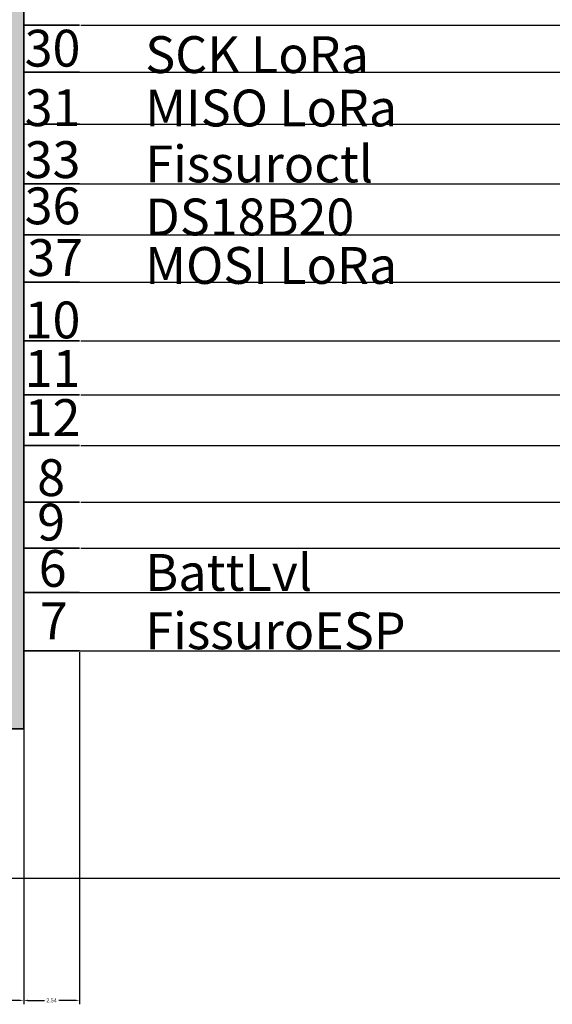
# Model space of a CAD drawing. Units: inches. Extents: x 23 to 132, y 5 to 105.
# Tile 7 of 14: x 81 to 105, y 5 to 50. Entities that reach past the tile are written whole.
import ezdxf

# ---------------------------------------------------------------- set-up
doc = ezdxf.new("R2010")
doc.units = ezdxf.units.IN
doc.header["$MEASUREMENT"] = 0
for name, color, linetype, lineweight in [('A-ANNO-DIMS', 2, 'Continuous', 18), ('E-ANNO-NETL', 30, 'Continuous', 18), ('E-ANNO-TEXT', 3, 'Continuous', 18), ('E-SYMB', 1, 'Continuous', 35), ('E-SYMB-PATT', 1, 'Continuous', 18), ('E-WIRE', 3, 'Continuous', 25)]:
    doc.layers.add(name, color=color, linetype=linetype, lineweight=lineweight)
doc.styles.get("Standard").update_dxf_attribs({"font": 'arial.ttf'})
doc.dimstyles.get("Standard").update_dxf_attribs({"dimtxt": 0.18, "dimasz": 0.18, "dimexe": 0.18, "dimexo": 0.0625, "dimgap": 0.09, "dimtad": 0, "dimtih": 1, "dimtoh": 1, "dimdec": 4, "dimzin": 0, "dimdsep": 46, "dimtxsty": 'Standard', "dimcen": 0.09, "dimadec": 0, "dimazin": 0, "dimtfac": 1, "dimtdec": 4, "dimtofl": 0, "dimtmove": 0, "dimatfit": 3, "dimfxl": 1, "dimtolj": 1, "dimtzin": 0, "dimarcsym": 0})

# ---------------------------------------------------------------- blocks, each defined once
blk = doc.blocks.new('*D3')
at = {"layer": 'A-ANNO-DIMS', "color": 0, "lineweight": -2, "transparency": 16777216}
for p, q in [((121.409, 99.285), (129.239, 99.285)), ((129.059, 99.105), (129.059, 55.423)), ((129.059, 11.378), (129.059, 55.06)), ((72.981, 11.198), (129.239, 11.198))]:
    blk.add_line(p, q, dxfattribs=at)
at = {"layer": 'A-ANNO-DIMS', "color": 0, "transparency": 16777216}
for points in [[(129.029, 99.105), (129.089, 99.105), (129.059, 99.285)], [(129.029, 11.378), (129.089, 11.378), (129.059, 11.198)]]:
    blk.add_solid(points, dxfattribs=at)
at = {"layer": 'Defpoints', "color": 0, "transparency": 16777216}
for p in [(121.346, 99.285), (129.059, 99.285), (72.919, 11.198)]:
    blk.add_point(p, dxfattribs=at)
at = {"layer": 'A-ANNO-DIMS', "color": 0, "transparency": 16777216, "insert": (129.059, 55.241), "char_height": 0.18, "attachment_point": 5}
blk.add_mtext('\\A1;88.09', dxfattribs=at)
blk = doc.blocks.new('*D4')
at = {"layer": 'A-ANNO-DIMS', "color": 0, "lineweight": -2, "transparency": 16777216}
for p, q in [((50.265, 17.944), (50.265, 5.443)), ((80.969, 17.944), (80.969, 5.443)), ((50.445, 5.623), (65.153, 5.623)), ((80.789, 5.623), (66.081, 5.623))]:
    blk.add_line(p, q, dxfattribs=at)
at = {"layer": 'A-ANNO-DIMS', "color": 0, "transparency": 16777216}
for points in [[(50.445, 5.653), (50.445, 5.593), (50.265, 5.623)], [(80.789, 5.653), (80.789, 5.593), (80.969, 5.623)]]:
    blk.add_solid(points, dxfattribs=at)
at = {"layer": 'Defpoints', "color": 0, "transparency": 16777216}
for p in [(50.265, 18.007), (80.969, 18.007), (80.969, 5.623)]:
    blk.add_point(p, dxfattribs=at)
at = {"layer": 'A-ANNO-DIMS', "color": 0, "transparency": 16777216, "insert": (65.617, 5.623), "char_height": 0.18, "attachment_point": 5}
blk.add_mtext('\\A1;30.705', dxfattribs=at)
blk = doc.blocks.new('*D14')
at = {"layer": 'A-ANNO-DIMS', "color": 0, "lineweight": -2, "transparency": 16777216}
for p, q in [((80.969, 21.494), (80.969, 5.443)), ((83.514, 21.494), (83.514, 5.443)), ((81.149, 5.623), (81.916, 5.623)), ((83.334, 5.623), (82.566, 5.623))]:
    blk.add_line(p, q, dxfattribs=at)
at = {"layer": 'A-ANNO-DIMS', "color": 0, "transparency": 16777216}
for points in [[(81.149, 5.653), (81.149, 5.593), (80.969, 5.623)], [(83.334, 5.653), (83.334, 5.593), (83.514, 5.623)]]:
    blk.add_solid(points, dxfattribs=at)
at = {"layer": 'Defpoints', "color": 0, "transparency": 16777216}
for p in [(80.969, 21.557), (83.514, 21.557), (83.514, 5.623)]:
    blk.add_point(p, dxfattribs=at)
at = {"layer": 'A-ANNO-DIMS', "color": 0, "transparency": 16777216, "insert": (82.241, 5.623), "char_height": 0.18, "attachment_point": 5}
blk.add_mtext('\\A1;2.54', dxfattribs=at)
blk = doc.blocks.new('*D35')
at = {"layer": 'A-ANNO-DIMS', "color": 0, "lineweight": -2, "transparency": 16777216}
for p, q in [((83.576, 52.617), (129.239, 52.617)), ((129.059, 52.437), (129.059, 51.532)), ((129.059, 50.264), (129.059, 51.168)), ((83.576, 50.084), (129.239, 50.084))]:
    blk.add_line(p, q, dxfattribs=at)
at = {"layer": 'A-ANNO-DIMS', "color": 0, "transparency": 16777216}
for points in [[(129.029, 52.437), (129.089, 52.437), (129.059, 52.617)], [(129.029, 50.264), (129.089, 50.264), (129.059, 50.084)]]:
    blk.add_solid(points, dxfattribs=at)
at = {"layer": 'Defpoints', "color": 0, "transparency": 16777216}
for p in [(83.514, 52.617), (83.514, 50.084), (129.059, 50.084)]:
    blk.add_point(p, dxfattribs=at)
at = {"layer": 'A-ANNO-DIMS', "color": 0, "transparency": 16777216, "insert": (129.059, 51.35), "char_height": 0.18, "attachment_point": 5}
blk.add_mtext('\\A1;2.53', dxfattribs=at)
blk = doc.blocks.new('*D36')
at = {"layer": 'A-ANNO-DIMS', "color": 0, "lineweight": -2, "transparency": 16777216}
for p, q in [((83.576, 50.084), (129.239, 50.084)), ((129.059, 49.904), (129.059, 49.198)), ((129.059, 48.129), (129.059, 48.834)), ((83.576, 47.949), (129.239, 47.949))]:
    blk.add_line(p, q, dxfattribs=at)
at = {"layer": 'A-ANNO-DIMS', "color": 0, "transparency": 16777216}
for points in [[(129.029, 49.904), (129.089, 49.904), (129.059, 50.084)], [(129.029, 48.129), (129.089, 48.129), (129.059, 47.949)]]:
    blk.add_solid(points, dxfattribs=at)
at = {"layer": 'Defpoints', "color": 0, "transparency": 16777216}
for p in [(83.514, 50.084), (83.514, 47.949), (129.059, 47.949)]:
    blk.add_point(p, dxfattribs=at)
at = {"layer": 'A-ANNO-DIMS', "color": 0, "transparency": 16777216, "insert": (129.059, 49.016), "char_height": 0.18, "attachment_point": 5}
blk.add_mtext('\\A1;2.13', dxfattribs=at)
blk = doc.blocks.new('*D37')
at = {"layer": 'A-ANNO-DIMS', "color": 0, "lineweight": -2, "transparency": 16777216}
for p, q in [((83.576, 47.949), (129.239, 47.949)), ((129.059, 47.769), (129.059, 46.946)), ((129.059, 45.759), (129.059, 46.582)), ((83.576, 45.579), (129.239, 45.579))]:
    blk.add_line(p, q, dxfattribs=at)
at = {"layer": 'A-ANNO-DIMS', "color": 0, "transparency": 16777216}
for points in [[(129.029, 47.769), (129.089, 47.769), (129.059, 47.949)], [(129.029, 45.759), (129.089, 45.759), (129.059, 45.579)]]:
    blk.add_solid(points, dxfattribs=at)
at = {"layer": 'Defpoints', "color": 0, "transparency": 16777216}
for p in [(83.514, 47.949), (83.514, 45.579), (129.059, 45.579)]:
    blk.add_point(p, dxfattribs=at)
at = {"layer": 'A-ANNO-DIMS', "color": 0, "transparency": 16777216, "insert": (129.059, 46.764), "char_height": 0.18, "attachment_point": 5}
blk.add_mtext('\\A1;2.37', dxfattribs=at)
blk = doc.blocks.new('*D38')
at = {"layer": 'A-ANNO-DIMS', "color": 0, "lineweight": -2, "transparency": 16777216}
for p, q in [((83.576, 45.579), (129.239, 45.579)), ((129.059, 45.399), (129.059, 44.398)), ((129.059, 43.037), (129.059, 44.037)), ((83.576, 42.857), (129.239, 42.857))]:
    blk.add_line(p, q, dxfattribs=at)
at = {"layer": 'A-ANNO-DIMS', "color": 0, "transparency": 16777216}
for points in [[(129.029, 45.399), (129.089, 45.399), (129.059, 45.579)], [(129.029, 43.037), (129.089, 43.037), (129.059, 42.857)]]:
    blk.add_solid(points, dxfattribs=at)
at = {"layer": 'Defpoints', "color": 0, "transparency": 16777216}
for p in [(83.514, 45.579), (83.514, 42.857), (129.059, 42.857)]:
    blk.add_point(p, dxfattribs=at)
at = {"layer": 'A-ANNO-DIMS', "color": 0, "transparency": 16777216, "insert": (129.059, 44.218), "char_height": 0.18, "attachment_point": 5}
blk.add_mtext('\\A1;2.722', dxfattribs=at)
blk = doc.blocks.new('*D39')
at = {"layer": 'A-ANNO-DIMS', "color": 0, "lineweight": -2, "transparency": 16777216}
for p, q in [((83.576, 42.857), (129.239, 42.857)), ((129.059, 42.677), (129.059, 41.877)), ((129.059, 40.714), (129.059, 41.513)), ((83.576, 40.534), (129.239, 40.534))]:
    blk.add_line(p, q, dxfattribs=at)
at = {"layer": 'A-ANNO-DIMS', "color": 0, "transparency": 16777216}
for points in [[(129.029, 42.677), (129.089, 42.677), (129.059, 42.857)], [(129.029, 40.714), (129.089, 40.714), (129.059, 40.534)]]:
    blk.add_solid(points, dxfattribs=at)
at = {"layer": 'Defpoints', "color": 0, "transparency": 16777216}
for p in [(83.514, 42.857), (83.514, 40.534), (129.059, 40.534)]:
    blk.add_point(p, dxfattribs=at)
at = {"layer": 'A-ANNO-DIMS', "color": 0, "transparency": 16777216, "insert": (129.059, 41.695), "char_height": 0.18, "attachment_point": 5}
blk.add_mtext('\\A1;2.32', dxfattribs=at)
blk = doc.blocks.new('*D40')
at = {"layer": 'A-ANNO-DIMS', "color": 0, "lineweight": -2, "transparency": 16777216}
for p, q in [((83.576, 40.534), (129.239, 40.534)), ((129.059, 40.354), (129.059, 39.637)), ((129.059, 38.555), (129.059, 39.273)), ((83.576, 38.375), (129.239, 38.375))]:
    blk.add_line(p, q, dxfattribs=at)
at = {"layer": 'A-ANNO-DIMS', "color": 0, "transparency": 16777216}
for points in [[(129.029, 40.354), (129.089, 40.354), (129.059, 40.534)], [(129.029, 38.555), (129.089, 38.555), (129.059, 38.375)]]:
    blk.add_solid(points, dxfattribs=at)
at = {"layer": 'Defpoints', "color": 0, "transparency": 16777216}
for p in [(83.514, 40.534), (83.514, 38.375), (129.059, 38.375)]:
    blk.add_point(p, dxfattribs=at)
at = {"layer": 'A-ANNO-DIMS', "color": 0, "transparency": 16777216, "insert": (129.059, 39.455), "char_height": 0.18, "attachment_point": 5}
blk.add_mtext('\\A1;2.159', dxfattribs=at)
blk = doc.blocks.new('*D41')
at = {"layer": 'A-ANNO-DIMS', "color": 0, "lineweight": -2, "transparency": 16777216}
for p, q in [((83.576, 38.375), (129.239, 38.375)), ((129.059, 38.195), (129.059, 37.219)), ((129.059, 35.88), (129.059, 36.856)), ((83.576, 35.7), (129.239, 35.7))]:
    blk.add_line(p, q, dxfattribs=at)
at = {"layer": 'A-ANNO-DIMS', "color": 0, "transparency": 16777216}
for points in [[(129.029, 38.195), (129.089, 38.195), (129.059, 38.375)], [(129.029, 35.88), (129.089, 35.88), (129.059, 35.7)]]:
    blk.add_solid(points, dxfattribs=at)
at = {"layer": 'Defpoints', "color": 0, "transparency": 16777216}
for p in [(83.514, 38.375), (83.514, 35.7), (129.059, 35.7)]:
    blk.add_point(p, dxfattribs=at)
at = {"layer": 'A-ANNO-DIMS', "color": 0, "transparency": 16777216, "insert": (129.059, 37.037), "char_height": 0.18, "attachment_point": 5}
blk.add_mtext('\\A1;2.68', dxfattribs=at)
blk = doc.blocks.new('*D42')
at = {"layer": 'A-ANNO-DIMS', "color": 0, "lineweight": -2, "transparency": 16777216}
for p, q in [((83.576, 35.7), (129.239, 35.7)), ((129.059, 35.52), (129.059, 34.65)), ((129.059, 33.417), (129.059, 34.286)), ((83.576, 33.237), (129.239, 33.237))]:
    blk.add_line(p, q, dxfattribs=at)
at = {"layer": 'A-ANNO-DIMS', "color": 0, "transparency": 16777216}
for points in [[(129.029, 35.52), (129.089, 35.52), (129.059, 35.7)], [(129.029, 33.417), (129.089, 33.417), (129.059, 33.237)]]:
    blk.add_solid(points, dxfattribs=at)
at = {"layer": 'Defpoints', "color": 0, "transparency": 16777216}
for p in [(83.514, 35.7), (83.514, 33.237), (129.059, 33.237)]:
    blk.add_point(p, dxfattribs=at)
at = {"layer": 'A-ANNO-DIMS', "color": 0, "transparency": 16777216, "insert": (129.059, 34.468), "char_height": 0.18, "attachment_point": 5}
blk.add_mtext('\\A1;2.463', dxfattribs=at)
blk = doc.blocks.new('*D43')
at = {"layer": 'A-ANNO-DIMS', "color": 0, "lineweight": -2, "transparency": 16777216}
for p, q in [((83.576, 33.237), (129.239, 33.237)), ((129.059, 33.057), (129.059, 32.259)), ((129.059, 31.097), (129.059, 31.895)), ((83.576, 30.917), (129.239, 30.917))]:
    blk.add_line(p, q, dxfattribs=at)
at = {"layer": 'A-ANNO-DIMS', "color": 0, "transparency": 16777216}
for points in [[(129.029, 33.057), (129.089, 33.057), (129.059, 33.237)], [(129.029, 31.097), (129.089, 31.097), (129.059, 30.917)]]:
    blk.add_solid(points, dxfattribs=at)
at = {"layer": 'Defpoints', "color": 0, "transparency": 16777216}
for p in [(83.514, 33.237), (83.514, 30.917), (129.059, 30.917)]:
    blk.add_point(p, dxfattribs=at)
at = {"layer": 'A-ANNO-DIMS', "color": 0, "transparency": 16777216, "insert": (129.059, 32.077), "char_height": 0.18, "attachment_point": 5}
blk.add_mtext('\\A1;2.32', dxfattribs=at)
blk = doc.blocks.new('*D44')
at = {"layer": 'A-ANNO-DIMS', "color": 0, "lineweight": -2, "transparency": 16777216}
for p, q in [((83.576, 30.917), (129.239, 30.917)), ((129.059, 30.737), (129.059, 29.808)), ((129.059, 28.515), (129.059, 29.444)), ((83.576, 28.335), (129.239, 28.335))]:
    blk.add_line(p, q, dxfattribs=at)
at = {"layer": 'A-ANNO-DIMS', "color": 0, "transparency": 16777216}
for points in [[(129.029, 30.737), (129.089, 30.737), (129.059, 30.917)], [(129.029, 28.515), (129.089, 28.515), (129.059, 28.335)]]:
    blk.add_solid(points, dxfattribs=at)
at = {"layer": 'Defpoints', "color": 0, "transparency": 16777216}
for p in [(83.514, 30.917), (83.514, 28.335), (129.059, 28.335)]:
    blk.add_point(p, dxfattribs=at)
at = {"layer": 'A-ANNO-DIMS', "color": 0, "transparency": 16777216, "insert": (129.059, 29.626), "char_height": 0.18, "attachment_point": 5}
blk.add_mtext('\\A1;2.582', dxfattribs=at)
blk = doc.blocks.new('*D45')
at = {"layer": 'A-ANNO-DIMS', "color": 0, "lineweight": -2, "transparency": 16777216}
for p, q in [((83.576, 28.335), (129.239, 28.335)), ((129.059, 28.155), (129.059, 27.473)), ((129.059, 26.427), (129.059, 27.109)), ((83.576, 26.247), (129.239, 26.247))]:
    blk.add_line(p, q, dxfattribs=at)
at = {"layer": 'A-ANNO-DIMS', "color": 0, "transparency": 16777216}
for points in [[(129.029, 28.155), (129.089, 28.155), (129.059, 28.335)], [(129.029, 26.427), (129.089, 26.427), (129.059, 26.247)]]:
    blk.add_solid(points, dxfattribs=at)
at = {"layer": 'Defpoints', "color": 0, "transparency": 16777216}
for p in [(83.514, 28.335), (83.514, 26.247), (129.059, 26.247)]:
    blk.add_point(p, dxfattribs=at)
at = {"layer": 'A-ANNO-DIMS', "color": 0, "transparency": 16777216, "insert": (129.059, 27.291), "char_height": 0.18, "attachment_point": 5}
blk.add_mtext('\\A1;2.09', dxfattribs=at)
blk = doc.blocks.new('*D46')
at = {"layer": 'A-ANNO-DIMS', "color": 0, "lineweight": -2, "transparency": 16777216}
for p, q in [((83.576, 26.247), (129.239, 26.247)), ((129.059, 26.067), (129.059, 25.419)), ((129.059, 24.408), (129.059, 25.055)), ((83.576, 24.228), (129.239, 24.228))]:
    blk.add_line(p, q, dxfattribs=at)
at = {"layer": 'A-ANNO-DIMS', "color": 0, "transparency": 16777216}
for points in [[(129.029, 26.067), (129.089, 26.067), (129.059, 26.247)], [(129.029, 24.408), (129.089, 24.408), (129.059, 24.228)]]:
    blk.add_solid(points, dxfattribs=at)
at = {"layer": 'Defpoints', "color": 0, "transparency": 16777216}
for p in [(83.514, 26.247), (83.514, 24.228), (129.059, 24.228)]:
    blk.add_point(p, dxfattribs=at)
at = {"layer": 'A-ANNO-DIMS', "color": 0, "transparency": 16777216, "insert": (129.059, 25.237), "char_height": 0.18, "attachment_point": 5}
blk.add_mtext('\\A1;2.02', dxfattribs=at)
blk = doc.blocks.new('*D47')
at = {"layer": 'A-ANNO-DIMS', "color": 0, "lineweight": -2, "transparency": 16777216}
for p, q in [((83.576, 24.228), (129.239, 24.228)), ((129.059, 24.048), (129.059, 23.074)), ((129.059, 21.737), (129.059, 22.71)), ((83.576, 21.557), (129.239, 21.557))]:
    blk.add_line(p, q, dxfattribs=at)
at = {"layer": 'A-ANNO-DIMS', "color": 0, "transparency": 16777216}
for points in [[(129.029, 24.048), (129.089, 24.048), (129.059, 24.228)], [(129.029, 21.737), (129.089, 21.737), (129.059, 21.557)]]:
    blk.add_solid(points, dxfattribs=at)
at = {"layer": 'Defpoints', "color": 0, "transparency": 16777216}
for p in [(83.514, 24.228), (83.514, 21.557), (129.059, 21.557)]:
    blk.add_point(p, dxfattribs=at)
at = {"layer": 'A-ANNO-DIMS', "color": 0, "transparency": 16777216, "insert": (129.059, 22.892), "char_height": 0.18, "attachment_point": 5}
blk.add_mtext('\\A1;2.67', dxfattribs=at)

msp = doc.modelspace()

# ---------------------------------------------------------------- hatches: boundary and pattern name
at = {"layer": 'E-SYMB-PATT'}
h = msp.add_hatch(color=256, dxfattribs=at)
h.dxf.hatch_style = 1
h.paths.add_polyline_path([(80.9692, 77.095), (50.2646, 77.095), (50.2646, 18.0066), (80.9692, 18.0066)])

# ---------------------------------------------------------------- linework, layer by layer
at = {"layer": 'E-SYMB'}
for p, q in [((80.9692, 50.0837), (83.5136, 50.0837)), ((80.9692, 47.949), (83.5136, 47.949)), ((80.9692, 45.5785), (83.5136, 45.5785)), ((80.9692, 42.8565), (83.5136, 42.8565)), ((80.9692, 40.5342), (83.5136, 40.5342)), ((80.9692, 38.3751), (83.5136, 38.3751)), ((80.9692, 35.6998), (83.5136, 35.6998)), ((80.9692, 33.2368), (83.5136, 33.2368)), ((80.9692, 30.917), (83.5136, 30.917)), ((80.9692, 28.3352), (83.5136, 28.3352)), ((80.9692, 26.2465), (83.5136, 26.2465)), ((80.9692, 24.2279), (83.5136, 24.2279)), ((80.9692, 21.5566), (83.5136, 21.5566))]:
    msp.add_line(p, q, dxfattribs=at)
msp.add_lwpolyline([(50.2646, 77.095), (80.9692, 77.095), (80.9692, 18.0066), (50.2646, 18.0066)], close=True, dxfattribs=at)
at = {"layer": 'E-WIRE'}
for p, q in [((83.5136, 47.949), (86.5493, 47.949)), ((83.5136, 45.5785), (86.5493, 45.5785)), ((83.5136, 42.8565), (86.5493, 42.8565)), ((83.5136, 40.5342), (86.5493, 40.5342)), ((83.5136, 38.3751), (86.5493, 38.3751)), ((83.5136, 24.2279), (86.5493, 24.2279)), ((83.5136, 21.5566), (86.5493, 21.5566))]:
    msp.add_line(p, q, dxfattribs=at)

# ---------------------------------------------------------------- texts
at = {"layer": 'E-ANNO-NETL'}
for s, p in [('SCK LoRa', (86.5135, 47.9078)), ('MISO LoRa', (86.5135, 45.4726)), ('Fissuroctl', (86.5135, 42.92)), ('DS18B20', (86.5135, 40.5048)), ('MOSI LoRa', (86.5135, 38.2935)), ('BattLvl', (86.5135, 24.296)), ('FissuroESP', (86.5135, 21.6325))]:
    msp.add_text(s, height=1.67943, dxfattribs=at).set_placement(p)
at = {"layer": 'E-ANNO-TEXT'}
for s, height, p in [('30', 1.67943, (81.0136, 48.2005)), ('31', 1.67943, (81.0136, 45.4874)), ('33', 1.67943, (81.0136, 43.1188)), ('36', 1.67943, (81.0136, 41.011)), ('37', 1.67943, (81.1285, 38.6529)), ('10', 1.67943, (81.0136, 35.8076)), ('11', 1.67943, (81.0136, 33.5963)), ('12', 1.67943, (81.0136, 31.3567)), ('8', 1.6794, (81.5845, 28.6181)), ('9', 1.6794, (81.5845, 26.5927)), ('6', 1.6794, (81.657, 24.4788)), ('7', 1.6794, (81.7054, 22.0877))]:
    msp.add_text(s, height=height, dxfattribs=at).set_placement(p)

# ---------------------------------------------------------------- dimensions: what is measured, and where the dimension line sits
at = {"layer": 'A-ANNO-DIMS'}
for base, p1, p2, override, picture, middle in [((129.0589, 99.2846), (72.9188, 11.1983), (121.3461, 99.2846), {"dimdec": 2, "dimlfac": 1, "dimrnd": 0, "dimzin": 0, "dimdsep": 46, "dimlunit": 2}, '*D3', (129.0589, 55.2415)), ((129.0589, 50.0837), (83.5136, 52.6172), (83.5136, 50.0837), {"dimdec": 2, "dimlfac": 1, "dimrnd": 0, "dimzin": 0, "dimdsep": 46, "dimlunit": 2}, '*D35', (129.0589, 51.3504)), ((129.0589, 47.949), (83.5136, 50.0837), (83.5136, 47.949), {"dimdec": 2, "dimlfac": 1, "dimrnd": 0, "dimzin": 0, "dimdsep": 46, "dimlunit": 2}, '*D36', (129.0589, 49.0163)), ((129.0589, 45.5785), (83.5136, 47.949), (83.5136, 45.5785), {"dimdec": 2, "dimlfac": 1, "dimrnd": 0, "dimzin": 0, "dimdsep": 46, "dimlunit": 2}, '*D37', (129.0589, 46.7637)), ((129.0589, 42.8565), (83.5136, 45.5785), (83.5136, 42.8565), {"dimdec": 3, "dimlfac": 1, "dimrnd": 0, "dimzin": 0, "dimdsep": 46, "dimlunit": 2}, '*D38', (129.0589, 44.2175)), ((129.0589, 40.5342), (83.5136, 42.8565), (83.5136, 40.5342), {"dimdec": 2, "dimlfac": 1, "dimrnd": 0, "dimzin": 0, "dimdsep": 46, "dimlunit": 2}, '*D39', (129.0589, 41.6954)), ((129.0589, 38.3751), (83.5136, 40.5342), (83.5136, 38.3751), {"dimdec": 3, "dimlfac": 1, "dimrnd": 0, "dimzin": 0, "dimdsep": 46, "dimlunit": 2}, '*D40', (129.0589, 39.4546)), ((129.0589, 35.6998), (83.5136, 38.3751), (83.5136, 35.6998), {"dimdec": 2, "dimlfac": 1, "dimrnd": 0, "dimzin": 0, "dimdsep": 46, "dimlunit": 2}, '*D41', (129.0589, 37.0375)), ((129.0589, 33.2368), (83.5136, 35.6998), (83.5136, 33.2368), {"dimdec": 3, "dimlfac": 1, "dimrnd": 0, "dimzin": 0, "dimdsep": 46, "dimlunit": 2}, '*D42', (129.0589, 34.4683)), ((129.0589, 30.917), (83.5136, 33.2368), (83.5136, 30.917), {"dimdec": 2, "dimlfac": 1, "dimrnd": 0, "dimzin": 0, "dimdsep": 46, "dimlunit": 2}, '*D43', (129.0589, 32.0769)), ((129.0589, 28.3352), (83.5136, 30.917), (83.5136, 28.3352), {"dimdec": 3, "dimlfac": 1, "dimrnd": 0, "dimzin": 0, "dimdsep": 46, "dimlunit": 2}, '*D44', (129.0589, 29.6261)), ((129.0589, 26.2465), (83.5136, 28.3352), (83.5136, 26.2465), {"dimdec": 2, "dimlfac": 1, "dimrnd": 0, "dimzin": 0, "dimdsep": 46, "dimlunit": 2}, '*D45', (129.0589, 27.2909)), ((129.0589, 24.2279), (83.5136, 26.2465), (83.5136, 24.2279), {"dimdec": 2, "dimlfac": 1, "dimrnd": 0, "dimzin": 0, "dimdsep": 46, "dimlunit": 2}, '*D46', (129.0589, 25.2372)), ((129.0589, 21.5566), (83.5136, 24.2279), (83.5136, 21.5566), {"dimdec": 2, "dimlfac": 1, "dimrnd": 0, "dimzin": 0, "dimdsep": 46, "dimlunit": 2}, '*D47', (129.0589, 22.8923))]:
    dim = msp.add_linear_dim(base=base, p1=p1, p2=p2, angle=90, dimstyle='Standard', override=override, dxfattribs=at)
    dim.commit()
    dim.dimension.update_dxf_attribs({"geometry": picture, "text_midpoint": middle})
for base, p1, p2, override, picture, middle in [((83.5136, 5.6233), (80.9692, 21.5566), (83.5136, 21.5566), {"dimdec": 2, "dimlfac": 1, "dimrnd": 0, "dimzin": 0, "dimdsep": 46, "dimlunit": 2}, '*D14', (82.2414, 5.6233)), ((80.9692, 5.6233), (50.2646, 18.0066), (80.9692, 18.0066), {"dimdec": 3, "dimlfac": 1, "dimrnd": 0, "dimzin": 0, "dimdsep": 46, "dimlunit": 2}, '*D4', (65.6169, 5.6233))]:
    dim = msp.add_linear_dim(base=base, p1=p1, p2=p2, dimstyle='Standard', override=override, dxfattribs=at)
    dim.commit()
    dim.dimension.update_dxf_attribs({"geometry": picture, "text_midpoint": middle})

doc.saveas('drawing.dxf')
